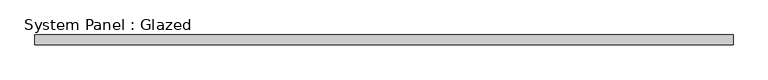
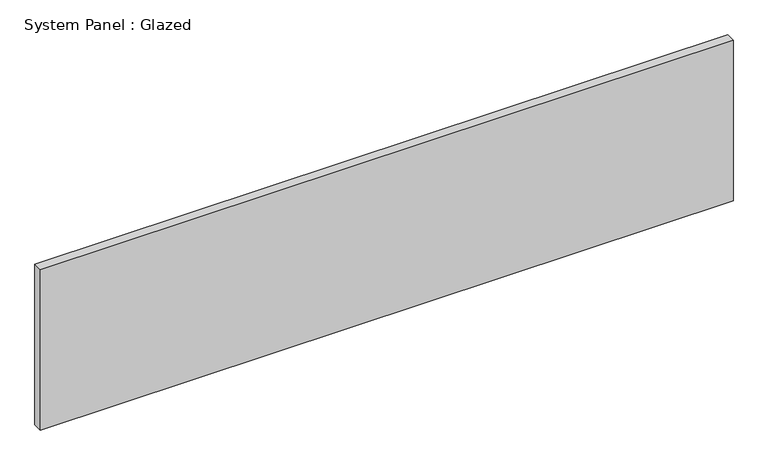
"""IFC4 building model written with IfcOpenShell, lengths in millimetres: plate geometry, System Panel : Glazed."""

from ifc_helpers import new_model, si_unit, origin, origin_with_axes, place, context, project, spatial, polyline, outline, extrude, source, transform, mapped, element, save


def system_panel_glazed_f495917c(model_context):
    return source(origin(), model_context, "Body", "SweptSolid", [
        extrude(outline(polyline([(917.575, 19.05), (-917.575, 19.05), (-917.575, 44.45), (917.575, 44.45), (917.575, 19.05)])), origin_with_axes(), (0.0, 0.0, 1.0), 448.8886718),
    ])


if __name__ == "__main__":
    model = new_model("IFC4")
    model_context = context("Model", 3, world=origin())
    ifc_project = project(units=[si_unit("LENGTHUNIT", "METRE", prefix="MILLI")], contexts=[model_context])
    site = spatial("IfcSite", under=ifc_project)
    building = spatial("IfcBuilding", under=site)
    placement = place(None, origin())
    system_panel_glazed_shape = system_panel_glazed_f495917c(model_context)
    element("IfcPlate", 1, ObjectType="System Panel : Glazed", at=placement, inside=building, context=model_context, shape_type="MappedRepresentation", body=[
        mapped(system_panel_glazed_shape, transform((0.0, 0.0, 0.0), x_axis=(1.0, 0.0, 0.0), y_axis=(0.0, 1.0, 0.0), z_axis=(0.0, 0.0, 1.0))),
    ])
    save(model, "model.ifc")

# Revit data of these elements
# Type "System Panel : Glazed"
#   Construction Type Id = "GSP4R"
#   Analytic Construction = "1/8 in Pilkington single glazing"
#   Visual Light Transmittance = 0.9
#   Solar Heat Gain Coefficient = 0.86
#   Heat Transfer Coefficient (U) = 1.18115 BTU/(h·ft²·°F)
#   Define Thermal Properties by = 1
# Element 1 (IfcPlate, "System Panel : Glazed")
#   Materials on its faces: "Glass"
# Materials
#   "Glass": class "Glass", colour RGB 0 128 192, transparency 0.75, Description = "Soda Lime Glass", Cost = 0
